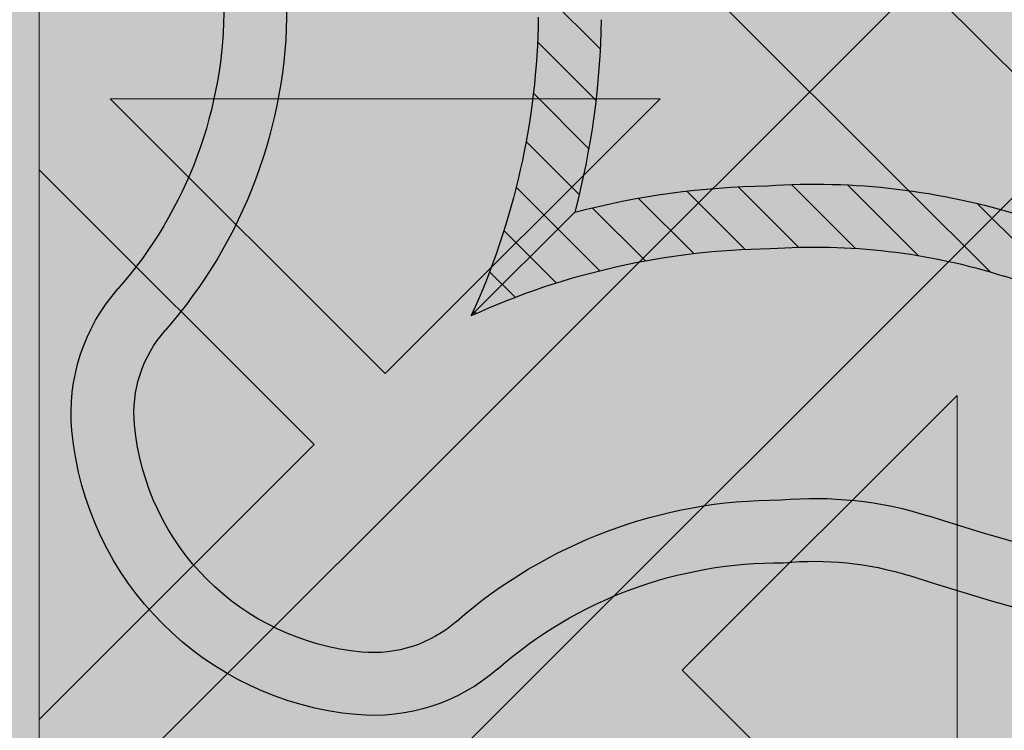
# Model space of a CAD drawing. Units: inches. Extents: x 844 to 2234, y 346 to 1084.
# Tile 28 of 93: x 1252.862 to 1255.358, y 687.38 to 689.183. Entities that reach past the tile are written whole.
import ezdxf

# ---------------------------------------------------------------- set-up
doc = ezdxf.new("R2010")
doc.units = ezdxf.units.IN
doc.header["$MEASUREMENT"] = 0
doc.layers.add('furniture', color=8, linetype='Continuous', lineweight=18)
doc.layers.add('RA-AP-01$0$INT', color=35, linetype='Continuous', lineweight=5)
doc.layers.add('RA-AP-01$0$FURN', color=3, linetype='Continuous')
doc.layers.add('RA-AP-01$0$WOOD', color=64, linetype='Continuous')

# ---------------------------------------------------------------- blocks, each defined once
blk = doc.blocks.new('A$C18D01794')
at = {"layer": 'RA-AP-01$0$INT'}
blk.add_hatch(color=256, dxfattribs=at).paths.add_polyline_path([(4.505206456958071, -6.306712009588038), (5.305206456958072, -6.306712009588038), (5.305206456958072, -7.106712009588038), (5.255206456951893, -7.10671200958804), (5.25520645694868, -6.356712009605972), (4.555206456959269, -6.356712009587461), (4.555206456956052, -7.106712009588038), (4.505206456958073, -7.106712009588038)])
h = blk.add_hatch(color=256, dxfattribs=at)
h.paths.add_polyline_path([(4.585917135068449, -6.356712009588271), (4.555206456959269, -6.35671200958746), (4.555206456959137, -6.387422687716308), (4.874495778835233, -6.706712009592356), (4.90520645695423, -6.676001331474049)])
h.paths.add_polyline_path([(5.255206456948813, -6.387422687716306), (5.255206456948682, -6.356712009605972), (5.224495778822613, -6.356712009605161), (4.905206456953498, -6.676001331474273), (4.935917135072151, -6.706712009592924)])
h.paths.add_polyline_path([(4.935917135072559, -6.706712009592068), (4.905206456953564, -6.737422687710376), (5.255206456951813, -7.087422687708613), (5.255206456951549, -7.026001331471008)])
h.paths.add_polyline_path([(4.555206456956399, -7.026001331471013), (4.555206456956134, -7.087422687708616), (4.905206456953821, -6.737422687710943), (4.874495778835166, -6.70671200959229)])
h = blk.add_hatch(color=256, dxfattribs=at)
h.paths.add_polyline_path([(4.585917135068448, -6.356712009588273), (4.614201406330596, -6.356712009589021), (4.668846067270487, -6.411356670531338), (4.723490728212344, -6.356712009591912), (4.771774999457151, -6.35671200959319), (4.826419660396886, -6.411356670535356), (4.862780050090322, -6.374996280843536), (4.844495778842715, -6.356712009595112), (4.862780050090411, -6.356712009595595), (4.905206456960182, -6.399138416468211), (4.947632863832445, -6.356712009597838), (4.965917135079675, -6.356712009598322), (4.947632863831759, -6.374996280845421), (4.983993253523576, -6.411356670538857), (5.038637914464627, -6.356712009600247), (5.08692218571208, -6.356712009601523), (5.141566846649976, -6.411356670541852), (5.196211507589851, -6.356712009604411), (5.224495778822615, -6.356712009605161), (4.905206456953975, -6.676001331473793)])
h.paths.add_polyline_path([(4.895206456956031, -6.637717060225675), (4.895206456958921, -6.528427738347902), (4.840561796018589, -6.583072399285802)], flags=16)
h.paths.add_polyline_path([(4.915206456955638, -6.637717060226121), (4.969851117895509, -6.583072399288678), (4.915206456957609, -6.528427738348344)], flags=16)
h.paths.add_polyline_path([(4.826419660395175, -6.568930263661755), (4.881064321335613, -6.514285602723745), (4.771774999456703, -6.514285602720857)], flags=16)
h.paths.add_polyline_path([(4.983993253519558, -6.568930263665262), (5.038637914460456, -6.514285602726792), (4.929348592581548, -6.514285602724816)], flags=16)
h.paths.add_polyline_path([(4.881064321336025, -6.494285602723742), (4.826419660397532, -6.439640941782821), (4.771774999457062, -6.494285602720859)], flags=16)
h.paths.add_polyline_path([(4.929348592582019, -6.494285602724817), (5.038637914460982, -6.494285602726792), (4.983993253522945, -6.439640941786327)], flags=16)
h.paths.add_polyline_path([(4.895206456960191, -6.480143467100443), (4.895206456962115, -6.407422687715913), (4.876922185715016, -6.389138416467584), (4.840561796021581, -6.425498806159401)], flags=16)
h.paths.add_polyline_path([(4.915206456958487, -6.480143467100889), (4.969851117899527, -6.425498806162279), (4.933490728206909, -6.389138416468043), (4.9152064569598, -6.40742268771434)], flags=16)
h.paths.add_polyline_path([(4.757632863832376, -6.480143467096812), (4.812277524772842, -6.425498806158772), (4.757632863834348, -6.370854145217844)], flags=16)
h.paths.add_polyline_path([(4.737632863832376, -6.480143467096286), (4.737632863834348, -6.370854145217375), (4.682988202893906, -6.425498806155385)], flags=16)
h.paths.add_polyline_path([(5.05278005008503, -6.480143467103376), (5.052780050087917, -6.370854145224413), (4.998135389146995, -6.425498806162908)], flags=16)
h.paths.add_polyline_path([(5.072780050085024, -6.480143467103744), (5.127424711025931, -6.42549880616527), (5.072780050087916, -6.370854145224832)], flags=16)
h.paths.add_polyline_path([(4.935917135072783, -6.706712009592292), (5.255206456948811, -6.387422687716309), (5.255206456948932, -6.415706958964177), (5.200561796010279, -6.470351619902839), (5.255206456949403, -6.524996280841948), (5.25520645694961, -6.5732805520894), (5.200561796009787, -6.627925213029239), (5.236922185702417, -6.664285602721864), (5.255206456949919, -6.646001331474357), (5.255206456949998, -6.664285602721898), (5.212780050078687, -6.706712009592262), (5.25520645695036, -6.749138416463932), (5.255206456950438, -6.767422687711313), (5.236922185702424, -6.749138416463297), (5.200561796009796, -6.785498806155928), (5.255206456950753, -6.840143467096874), (5.25520645695096, -6.888427738341682), (5.200561796010322, -6.943072399282328), (5.255206456951428, -6.997717060223427), (5.255206456951547, -7.026001331471006)])
h.paths.add_polyline_path([(5.042988202883395, -6.785498806155427), (5.097632863823085, -6.840143467095101), (5.097632863822622, -6.730854145216193)], flags=16)
h.paths.add_polyline_path([(5.028846067259663, -6.771356670531693), (5.083490728198774, -6.716712009592573), (4.974201406321001, -6.716712009593042)], flags=16)
h.paths.add_polyline_path([(5.117632863823087, -6.840143467095186), (5.172277524762331, -6.785498806155926), (5.11763286382262, -6.730854145216225)], flags=16)
h.paths.add_polyline_path([(5.08349072819877, -6.696712009593886), (5.028846067259652, -6.642067348654775), (4.974201406320998, -6.696712009593438)], flags=16)
h.paths.add_polyline_path([(5.131774999446817, -6.854285602718917), (5.186419660386065, -6.799640941779662), (5.241064321325782, -6.854285602719365)], flags=17)
h.paths.add_polyline_path([(5.131774999446228, -6.716712009592374), (5.186419660386065, -6.771356670532194), (5.222780050079488, -6.734996280838764), (5.204495778832781, -6.716712009592063)], flags=16)
h.paths.add_polyline_path([(5.097632863822613, -6.682569873970264), (5.097632863823061, -6.573280552091354), (5.042988202883383, -6.627925213031044)], flags=16)
h.paths.add_polyline_path([(5.131774999446899, -6.874285602718915), (5.241064321325809, -6.874285602719364), (5.186419660386591, -6.928930263658598)], flags=17)
h.paths.add_polyline_path([(5.131774999446226, -6.696712009594078), (5.204495778830767, -6.696712009594374), (5.22278005007868, -6.67842773834687), (5.186419660386049, -6.642067348654249)], flags=16)
h.paths.add_polyline_path([(5.11763286382262, -6.682569873970225), (5.17227752476232, -6.627925213030515), (5.117632863823064, -6.573280552091267)], flags=16)
h.paths.add_polyline_path([(5.186419660386069, -6.613783077405491), (5.241064321325754, -6.559138416465795), (5.131774999446791, -6.559138416466263)], flags=16)
h.paths.add_polyline_path([(5.131774999446872, -6.539138416466263), (5.24106432132578, -6.539138416465794), (5.186419660386554, -6.484493755526573)], flags=16)
h.paths.add_polyline_path([(5.255206456951811, -7.08742268770861), (5.255206456951895, -7.106712009588038), (4.555206456956052, -7.106712009588038), (4.555206456956136, -7.087422687708617), (4.905206456953973, -6.737422687710788)])
h.paths.add_polyline_path([(4.983993253513404, -6.8444937555241), (4.92934859257295, -6.899138416462108), (5.03863791445186, -6.899138416465014)], flags=16)
h.paths.add_polyline_path([(4.969851117889988, -6.83035161990006), (4.915206456952556, -6.775706958960171), (4.915206456949648, -6.884996280837944)], flags=16)
h.paths.add_polyline_path([(4.929348592572535, -6.919138416462105), (4.983993253511019, -6.973783077403037), (5.038637914451496, -6.919138416465012)], flags=16)
h.paths.add_polyline_path([(5.052780050074912, -6.93328055208906), (4.998135389134438, -6.987925213027088), (5.052780050072919, -7.042569873968025)], flags=16)
h.paths.add_polyline_path([(5.07278005007491, -6.933280552089588), (5.072780050072918, -7.042569873968497), (5.127424711013374, -6.987925213030498)], flags=16)
h.paths.add_polyline_path([(4.89520645695295, -6.775706958959721), (4.840561796013067, -6.830351619897157), (4.895206456950961, -6.884996280837494)], flags=16)
h.paths.add_polyline_path([(4.915206456948365, -6.933280552085403), (4.915206456946434, -7.006001331471951), (4.933490728192729, -7.024285602719066), (4.969851117886972, -6.987925213026453)], flags=16)
h.paths.add_polyline_path([(4.881064321327021, -6.899138416461022), (4.82641966038902, -6.84449375552057), (4.771774999448108, -6.899138416459029)], flags=16)
h.paths.add_polyline_path([(4.895206456950073, -6.933280552084951), (4.840561796009022, -6.987925213023558), (4.876922185700835, -7.024285602716997), (4.895206456948749, -7.006001331469487)], flags=16)
h.paths.add_polyline_path([(4.983993253510392, -7.0020673486505), (4.947632863816944, -7.038427738342319), (4.965917135064043, -7.05671200959023), (5.038637914448995, -7.056712009591555)], flags=16)
h.paths.add_polyline_path([(4.881064321326543, -6.91913841646102), (4.771774999447578, -6.919138416459031), (4.826419660385607, -6.973783077399508)], flags=16)
h.paths.add_polyline_path([(4.905206456946447, -7.014285602717636), (4.862780050074785, -7.056712009588352), (4.947632863816685, -7.056712009589775)], flags=16)
h.paths.add_polyline_path([(5.14156684663679, -7.002067348654549), (5.086922185696452, -7.056712009592438), (5.196211507574223, -7.056712009594425)], flags=16)
h.paths.add_polyline_path([(4.8264196603837, -7.002067348646972), (4.771774999442643, -7.056712009585575), (4.8444957788276, -7.056712009587508), (4.862780050075511, -7.038427738340416)], flags=16)
h.paths.add_polyline_path([(4.812277524760289, -6.98792521302292), (4.757632863822258, -6.933280552082447), (4.757632863819352, -7.042569873961408)], flags=16)
h.paths.add_polyline_path([(4.73763286382226, -6.933280552082079), (4.682988202881349, -6.987925213020536), (4.737632863819352, -7.04256987396099)], flags=16)
h.paths.add_polyline_path([(4.723490728195188, -7.056712009584289), (4.668846067257299, -7.002067348643949), (4.614201406317417, -7.056712009581383)], flags=16)
h.paths.add_polyline_path([(4.597632863829262, -6.706712009592262), (4.555206456957951, -6.664285602721896), (4.555206456958029, -6.646001331474357), (4.573490728205535, -6.664285602721864), (4.609851117898167, -6.627925213029238), (4.555206456958338, -6.573280552089402), (4.555206456958546, -6.524996280841952), (4.60985111789767, -6.470351619902839), (4.555206456959015, -6.415706958964177), (4.555206456959138, -6.387422687716309), (4.874495778835167, -6.70671200959229), (4.5552064569564, -7.026001331471015), (4.555206456956523, -6.997717060223433), (4.609851117897629, -6.94307239928233), (4.555206456956988, -6.888427738341681), (4.555206456957198, -6.840143467096881), (4.609851117898153, -6.78549880615593), (4.573490728205528, -6.749138416463297), (4.555206456957507, -6.76742268771132), (4.555206456957585, -6.749138416463933)])
h.paths.add_polyline_path([(4.712780050085332, -6.730854145216195), (4.712780050084863, -6.840143467095105), (4.767424711024555, -6.785498806155427)], flags=16)
h.paths.add_polyline_path([(4.726922185709173, -6.716712009592573), (4.781566846648288, -6.771356670531693), (4.836211507586949, -6.716712009593043)], flags=16)
h.paths.add_polyline_path([(4.692780050085327, -6.730854145216225), (4.638135389145619, -6.785498806155928), (4.692780050084865, -6.840143467095185)], flags=16)
h.paths.add_polyline_path([(4.726922185709182, -6.696712009593886), (4.836211507586949, -6.696712009593436), (4.7815668466483, -6.642067348654773)], flags=16)
h.paths.add_polyline_path([(4.678637914461726, -6.71671200959237), (4.605917135075169, -6.716712009592063), (4.587632863828464, -6.734996280838766), (4.623993253521887, -6.771356670532195)], flags=16)
h.paths.add_polyline_path([(4.712780050085336, -6.68256987397026), (4.767424711024568, -6.627925213031042), (4.71278005008489, -6.573280552091352)], flags=16)
h.paths.add_polyline_path([(4.678637914461726, -6.696712009594076), (4.623993253521899, -6.642067348654247), (4.587632863829271, -6.67842773834687), (4.605917135077185, -6.696712009594376)], flags=16)
h.paths.add_polyline_path([(4.692780050085336, -6.682569873970228), (4.692780050084889, -6.573280552091267), (4.638135389145632, -6.627925213030515)], flags=16)
h.paths.add_polyline_path([(4.623993253521885, -6.799640941779662), (4.678637914461131, -6.854285602718915), (4.56934859258217, -6.854285602719365)], flags=17)
h.paths.add_polyline_path([(4.623993253521901, -6.613783077405509), (4.678637914461158, -6.559138416466263), (4.569348592582195, -6.559138416465795)], flags=16)
h.paths.add_polyline_path([(4.678637914461051, -6.874285602718915), (4.623993253521361, -6.928930263658598), (4.569348592582143, -6.874285602719364)], flags=17)
h.paths.add_polyline_path([(4.678637914461076, -6.539138416466263), (4.623993253521399, -6.484493755526573), (4.569348592582167, -6.539138416465796)], flags=16)
h = blk.add_hatch(color=256, dxfattribs=at)
h.paths.add_polyline_path([(4.969851117891331, -6.583072399286455), (4.915206456952669, -6.63771706022511), (4.915206456952222, -6.528427738347337)])
h.paths.add_polyline_path([(4.895206456953064, -6.637717060225108), (4.840561796014413, -6.583072399286448), (4.895206456953533, -6.528427738347335)])
h.paths.add_polyline_path([(4.826419660390684, -6.568930263662714), (4.771774999451003, -6.514285602723024), (4.881064321329913, -6.514285602723489)])
h.paths.add_polyline_path([(4.881064321329884, -6.494285602723492), (4.771774999450921, -6.494285602723024), (4.82641966039018, -6.439640941783778)])
h.paths.add_polyline_path([(4.895206456953734, -6.48014346709988), (4.840561796013912, -6.425498806160046), (4.876922185707337, -6.389138416466622), (4.895206456954043, -6.40742268771333)])
h.paths.add_polyline_path([(4.862780050082808, -6.374996280843689), (4.826419660390178, -6.411356670536314), (4.771774999450351, -6.356712009596481), (4.844495778835303, -6.356712009596181)])
h.paths.add_polyline_path([(4.812277524766446, -6.425498806160041), (4.757632863827191, -6.480143467099289), (4.757632863826741, -6.370854145220329)])
h.paths.add_polyline_path([(4.737632863827191, -6.480143467099214), (4.682988202887508, -6.425498806159518), (4.737632863826743, -6.370854145220299)])
h.paths.add_polyline_path([(4.668846067263777, -6.41135667053579), (4.614201406325123, -6.356712009597128), (4.723490728202894, -6.356712009596675)])
h.paths.add_polyline_path([(4.905206456953846, -6.399138416467422), (4.862780050082654, -6.356712009596229), (4.947632863824561, -6.356712009595756)])
h.paths.add_polyline_path([(4.915206456952028, -6.480143467099882), (4.91520645695173, -6.407422687715346), (4.933490728199234, -6.389138416467428), (4.96985111789186, -6.425498806160055)])
h.paths.add_polyline_path([(5.038637914454841, -6.494285602723048), (4.929348592575874, -6.494285602723497), (4.983993253515593, -6.439640941783787)])
h.paths.add_polyline_path([(4.983993253515065, -6.568930263662725), (4.929348592575849, -6.514285602723495), (5.038637914454755, -6.514285602723045)])
h.paths.add_polyline_path([(5.052780050079843, -6.480143467099317), (4.998135389140595, -6.425498806160058), (5.052780050080309, -6.370854145220356)])
h.paths.add_polyline_path([(4.983993253516868, -6.411356670536324), (4.947632863824241, -6.374996280843694), (4.965917135071747, -6.356712009596188), (5.038637914456701, -6.356712009596504)])
h.paths.add_polyline_path([(5.127424711019533, -6.425498806159557), (5.072780050079843, -6.480143467099239), (5.07278005008031, -6.370854145220326)])
h.paths.add_polyline_path([(5.141566846643269, -6.411356670535829), (5.086922185704154, -6.356712009596707), (5.196211507581929, -6.356712009597176)])
h = blk.add_hatch(color=256, dxfattribs=at)
h.paths.add_polyline_path([(5.028846067259997, -6.642067348655121), (4.974201406321342, -6.696712009593783), (5.083490728199115, -6.69671200959423)])
h.paths.add_polyline_path([(4.974201406321344, -6.716712009593388), (5.028846067260004, -6.771356670532039), (5.083490728199117, -6.716712009592919)])
h.paths.add_polyline_path([(5.042988202883738, -6.785498806155768), (5.097632863823428, -6.840143467095449), (5.097632863822963, -6.73085414521654)])
h.paths.add_polyline_path([(5.117632863822961, -6.730854145216568), (5.117632863823428, -6.840143467095531), (5.172277524762674, -6.785498806156272)])
h.paths.add_polyline_path([(5.131774999446572, -6.716712009592718), (5.186419660386406, -6.77135667053254), (5.222780050079831, -6.734996280839116), (5.204495778833122, -6.716712009592409)])
h.paths.add_polyline_path([(5.236922185702764, -6.749138416463644), (5.200561796010139, -6.785498806156274), (5.255206456949971, -6.840143467096101), (5.255206456950271, -6.76742268771115)])
h.paths.add_polyline_path([(5.186419660386412, -6.799640941780006), (5.131774999447164, -6.854285602719262), (5.241064321326123, -6.854285602719711)])
h.paths.add_polyline_path([(5.131774999447238, -6.874285602719261), (5.186419660386934, -6.928930263658944), (5.241064321326153, -6.874285602719709)])
h.paths.add_polyline_path([(5.200561796010663, -6.943072399282675), (5.255206456949324, -6.997717060221329), (5.255206456949777, -6.888427738343558)])
h.paths.add_polyline_path([(5.21278005007903, -6.706712009592607), (5.255206456950223, -6.749138416463798), (5.255206456950696, -6.664285602721891)])
h.paths.add_polyline_path([(5.13177499944657, -6.696712009594424), (5.204495778831106, -6.696712009594723), (5.222780050079024, -6.678427738347219), (5.186419660386397, -6.642067348654592)])
h.paths.add_polyline_path([(5.117632863823405, -6.573280552091611), (5.117632863822955, -6.682569873970578), (5.172277524762665, -6.627925213030859)])
h.paths.add_polyline_path([(5.042988202883727, -6.627925213031387), (5.097632863822957, -6.682569873970603), (5.097632863823407, -6.573280552091697)])
h.paths.add_polyline_path([(5.131774999447135, -6.559138416466609), (5.186419660386394, -6.613783077405857), (5.241064321326097, -6.559138416466144)])
h.paths.add_polyline_path([(5.200561796010128, -6.627925213029584), (5.236922185702758, -6.664285602722211), (5.255206456950264, -6.646001331474705), (5.255206456949948, -6.573280552089752)])
h.paths.add_polyline_path([(5.186419660386895, -6.484493755526919), (5.131774999447213, -6.539138416466609), (5.241064321326127, -6.539138416466142)])
h.paths.add_polyline_path([(5.200561796010624, -6.470351619903183), (5.255206456949745, -6.524996280842298), (5.255206456949276, -6.415706958964523)])
for p, q in [((4.905206456953975, -6.676001331473793), (5.224495778822613, -6.356712009605161)), ((5.255206456951895, -7.106712009588038), (5.255206456948681, -6.356712009605972)), ((5.072780050085028, -6.48014346710374), (5.072780050087916, -6.37085414522483)), ((5.072780050087916, -6.37085414522483), (5.127424711025931, -6.42549880616527)), ((4.935917135072783, -6.706712009592292), (5.255206456948813, -6.387422687716307)), ((5.255206456948934, -6.415706958964177), (5.200561796010281, -6.470351619902839)), ((5.12742471102593, -6.425498806165272), (5.072780050085028, -6.48014346710374)), ((5.255206456949399, -6.524996280841946), (5.200561796010281, -6.470351619902839)), ((5.18641966038655, -6.484493755526575), (5.131774999446872, -6.539138416466263)), ((5.241064321325782, -6.539138416465796), (5.186419660386552, -6.484493755526573)), ((5.131774999446872, -6.539138416466263), (5.241064321325782, -6.539138416465796))]:
    blk.add_line(p, q, dxfattribs=at)
blk = doc.blocks.new('A$C32926AE1')
at = {"layer": 'RA-AP-01$0$FURN'}
h = blk.add_hatch(dxfattribs=at)
h.set_pattern_fill('ANSI31', color=256, scale=0.1, style=0)
h.set_pattern_definition([(45, (0, 0), (-0.0088388347648318, 0.0088388347648318), [])])
edge = h.paths.add_edge_path(flags=16)
edge.add_arc((4.904771284329206, 4.246793130718756), 0.2603971832811541, 75.22398030683196, 104.7760196931204)
edge.add_arc((4.904771284329206, 4.246793130718756), 0.2603971832811541, 75.223980306832, 104.77601969312039, ccw=False)
edge = h.paths.add_edge_path(flags=16)
edge.add_arc((4.904771284329206, 4.067062675376612), 0.2603971832811541, 255.2239803068796, 284.776019693168)
edge.add_arc((4.904771284329206, 4.067062675376612), 0.2603971832811541, 255.22398030687958, 284.77601969316805, ccw=False)
edge = h.paths.add_edge_path(flags=0)
edge.add_arc((4.904771284329206, 4.067062675376612), 0.2603971832811541, 255.2239803068796, 284.776019693168)
edge.add_arc((4.904771284329206, 4.067062675376612), 0.2603971832811541, 255.22398030687958, 284.77601969316805, ccw=False)
edge = h.paths.add_edge_path(flags=0)
edge.add_arc((4.904771284329206, 4.067062675376612), 0.2603971832811541, 255.2239803068796, 284.776019693168)
edge.add_arc((4.904771284329206, 4.067062675376612), 0.2603971832811541, 255.22398030687958, 284.77601969316805, ccw=False)
edge = h.paths.add_edge_path()
edge.add_arc((4.604388392048174, 4.588829985554312), 0.1599999999999918, 342.3781640246255, 354.4317409793762)
edge.add_arc((5.090145208887507, 4.43216705527679), 0.3503971832811637, 162.0091218307731, 180.3186872093483)
edge.add_arc((5.205154176610243, 4.588829985554953), 0.1599999999999917, 185.5682590208461, 197.6218359767349)
edge.add_arc((4.904771284329229, 4.246793130718735), 0.3503971832811761, 72.00912183053516, 107.9908781690354)
edge.add_arc((9.535952835716557, 4.28682295566602), 4.798342501046485, 178.2875002453811, 181.5576802719453)
edge.add_arc((4.719397359771122, 4.43216705527679), 0.3503971832811637, 359.6813127906516, 377.9908781692269)
edge.add_arc((9.535967292294904, 4.286822350292874), 4.778371420254705, 178.2965938931842, 181.5667745797229)
edge.add_arc((4.719397359771122, 4.43216705527679), 0.3303971832811637, 359.6813127906516, 377.9908781692269)
edge.add_arc((0.2735752763637294, 4.286822350292874), 4.7783714202547, 358.4332254202771, 361.7034061068158)
edge.add_arc((5.061434214606998, 4.732549947558029), 0.1600000000000254, 252.3781640250584, 264.4317409792362)
edge.add_arc((4.748108354051257, 4.732549947558012), 0.1600000000000541, 275.5682590208426, 287.6218359759532)
edge.add_arc((4.604388392048115, 4.588829985554317), 0.1800000000000505, 342.3567572500182, 349.3735009646207)
edge.add_arc((5.205154176610254, 4.588829985554976), 0.1800000000000069, 190.6264990356027, 197.6432427513933)
edge.add_arc((5.061434214607106, 4.732549947558013), 0.1800000000000424, 252.3567572496606, 259.3735009644582)
edge.add_arc((4.904771284329208, 4.246793130718737), 0.3303971832811676, 71.99844483668534, 108.0015551637021)
edge.add_arc((4.748108354051414, 4.732549947558045), 0.1800000000000547, 280.6264990355479, 287.6432427495938)
edge.add_arc((5.090145208887514, 4.432167055276789), 0.2803971832811691, 162.8706300666893, 180.816523289902)
edge.add_arc((4.719397359771136, 4.432167055276689), 0.2803971832811534, 359.183476710103, 377.1293699333214)
edge.add_arc((4.904771284329222, 4.246793130718737), 0.2803971832811769, 72.87063006672916, 107.1293699332334)
edge.add_arc((5.090145208887522, 4.432167055276788), 0.2603971832811776, 165.2239803068007, 180.9953123810312)
edge.add_arc((4.719397359771141, 4.432167055276699), 0.2603971832811458, 359.0046876189768, 374.7760196932087)
edge.add_arc((5.090145208887507, 4.43216705527679), 0.3303971832811637, 162.0091218307731, 180.3186872093483)
edge.add_arc((9.53595427642584, 4.285015535491528), 4.728345371032053, 178.265043920078, 181.5679956281801)
edge.add_arc((0.2735882922327999, 4.285015535491582), 4.728345371032045, 358.4320043718193, 361.7349560799204)
edge.add_arc((9.535953591267507, 4.284458026472751), 4.708343996644348, 178.2573054306777, 181.5704995759608)
edge.add_arc((0.273588977391114, 4.284458026472785), 4.708343996644358, 358.4295004240388, 361.7426945693213)
edge.add_arc((0.2735889773911131, 4.029397779622582), 4.708343996644359, 358.2573054306787, 361.5704995759613)
edge.add_arc((9.535953591267518, 4.029397779622618), 4.708343996644359, 178.4295004240391, 181.7426945693223)
edge.add_arc((0.2735882922327901, 4.028840270603786), 4.728345371032054, 358.2650439200796, 361.5679956281808)
edge.add_arc((9.53595427642584, 4.028840270603841), 4.728345371032054, 178.4320043718199, 181.7349560799219)
edge.add_arc((0.2735752763637302, 4.027033455802493), 4.778371420254699, 358.2965938931842, 361.5667745797229)
edge.add_arc((4.719397359771122, 3.881688750818578), 0.3303971832811637, 342.0091218307731, 360.3186872093484)
edge.add_arc((5.090145208887507, 3.881688750818578), 0.3303971832811637, 179.6813127906516, 197.9908781692269)
edge.add_arc((9.535967292294904, 4.027033455802493), 4.778371420254705, 178.433225420277, 181.7034061068158)
edge.add_arc((4.719397359771122, 3.881688750818578), 0.3503971832811637, 342.0091218307731, 360.3186872093484)
edge.add_arc((9.53595283571655, 4.027032850429349), 4.79834250104648, 178.4423197280546, 181.7124997546188)
edge.add_arc((4.719397359771141, 3.881688750818669), 0.2603971832811458, 345.2239803067913, 360.9953123810232)
edge.add_arc((5.090145208887522, 3.88168875081858), 0.2603971832811776, 179.0046876189687, 194.7760196931993)
edge.add_arc((4.904771284329222, 4.067062675376631), 0.2803971832811769, 252.8706300667665, 287.1293699332708)
edge.add_arc((4.719397359771136, 3.881688750818678), 0.2803971832811534, 342.8706300666787, 360.8165232898969)
edge.add_arc((5.090145208887514, 3.881688750818579), 0.2803971832811691, 179.183476710098, 197.1293699333106)
edge.add_arc((4.748108354051414, 3.581305858537323), 0.1800000000000547, 72.3567572504062, 79.37350096445199)
edge.add_arc((4.904771284329208, 4.067062675376631), 0.3303971832811676, 251.9984448362979, 288.0015551633146)
edge.add_arc((5.061434214607106, 3.581305858537355), 0.1800000000000424, 100.6264990355418, 107.6432427503394)
edge.add_arc((5.205154176610254, 3.725025820540392), 0.1800000000000069, 162.3567572486066, 169.3735009643972)
edge.add_arc((4.604388392048115, 3.725025820541051), 0.1800000000000505, 10.62649903537925, 17.64324274998182)
edge.add_arc((4.748108354051257, 3.581305858537356), 0.1600000000000541, 72.37816402404681, 84.43174097915735)
edge.add_arc((4.904771284329229, 4.067062675376632), 0.3503971832811761, 252.0091218309645, 287.9908781694648)
edge.add_arc((5.061434214606998, 3.581305858537339), 0.1600000000000254, 95.56825902076373, 107.6218359749416)
edge.add_arc((5.205154176610243, 3.725025820540414), 0.1599999999999917, 162.3781640232651, 174.4317409791539)
edge.add_arc((5.090145208887507, 3.881688750818578), 0.3503971832811637, 179.6813127906516, 197.9908781692269)
edge.add_arc((4.604388392048174, 3.725025820541056), 0.1599999999999918, 5.568259020623824, 17.62183597537444)
edge.add_arc((0.2735897329420762, 4.28682295566602), 4.798342501046482, 358.4423197280547, 361.7124997546188)
edge.add_arc((0.2735897329420691, 4.027032850429348), 4.798342501046489, 358.2875002453812, 361.5576802719453)
at = {"layer": 'RA-AP-01$0$WOOD'}
h = blk.add_hatch(color=256, dxfattribs=at)
h.dxf.hatch_style = 1
h.paths.add_polyline_path([(5.157430609644524, 4.573483066760929, -0.1009492694046607), (5.155401577623758, 4.593365984175333, -0.1842662638101597), (5.172249623284174, 4.638795604568598, 0.2056608120311276), (5.179560981299304, 4.661316324430096, 0.3614336704623542), (5.134352340494423, 4.706524965234944, 0.2056608120311297), (5.111831620632933, 4.699213607219793, -0.1842662638101113), (5.066402000239693, 4.682365561559342, -0.1055311479399994), (5.045656153913092, 4.68467289944697, 0.1567636581983829), (4.763886414745334, 4.684672899446966, -0.1055311479399895), (4.743140568418733, 4.68236556155934, -0.1842662638100833), (4.6977109480255, 4.69921360721979, 0.2056608120302612), (4.675190228164109, 4.706524965234949, 0.3614336704708441), (4.629981587358889, 4.66131632442871, 0.2056608120245944), (4.637292945374126, 4.638795604567974, -0.1842662638101024), (4.654140991034615, 4.59336598417475, -0.1009492694055169), (4.652111959013835, 4.573483066760181, 0.021410119221476), (4.629748025606143, 4.156712009541676, 0.0214101192214795), (4.652111959013809, 3.739940952323101, -0.1009492694059586), (4.654140991034615, 3.720058034908448, -0.1842662638100975), (4.637292945374126, 3.674628414515226, 0.2056608120245705), (4.629981587358889, 3.652107694654492, 0.3614336704708879), (4.675190228164113, 3.606899053848249, 0.2056608120302384), (4.697710948025501, 3.614210411863408, -0.1842662638100995), (4.743140568418738, 3.63105845752386, -0.1055311479402541), (4.763886414745388, 3.628751119636215, 0.1567636581983776), (5.045656153913137, 3.628751119636244, -0.1055311479397538), (5.066402000239692, 3.631058457523857, -0.1842662638101067), (5.111831620632931, 3.614210411863407, 0.2056608120310924), (5.134352340494417, 3.606899053848256, 0.3614336704624001), (5.179560981299307, 3.652107694653103, 0.2056608120311314), (5.172249623284175, 3.6746284145146, -0.1842662638101402), (5.155401577623758, 3.72005803490786, -0.1009492694051366), (5.15743060964455, 3.739940952322354, 0.0214101192215073), (5.179794543052287, 4.156712009541468, 0.0214101192215252)])
h.paths.add_polyline_path([(4.639748609479751, 4.156712009541513, 0.0213537860821624), (4.661970494867118, 3.741887061152232, -0.094075836301374), (4.664143710413708, 3.7196126951003, -0.1824818158568985), (4.644813765429836, 3.668037719127816, 0.2056608120245319), (4.639939526753007, 3.653023905887301, 0.3614336704710246), (4.676106439397173, 3.616856993242342, 0.2056608120302234), (4.691120252638095, 3.621731231919122, -0.1824818158602558), (4.742695228611606, 3.641061176902986, -0.1029891339458722), (4.766991894714349, 3.638256818950944, 0.156709409989566), (5.042550673941472, 3.638256818950105, -0.102989133958497), (5.066847340047078, 3.641061176902949, -0.1824818158594995), (5.118422316020358, 3.621731231919103, 0.2056608120311416), (5.133436129261316, 3.616856993242346, 0.3614336704621468), (5.169603041905217, 3.653023905886178, 0.2056608120310986), (5.164728803228477, 3.668037719127177, -0.1824818158565612), (5.145398858244737, 3.719612695099578, -0.0940758363009313), (5.147572073791232, 3.741887061151398, 0.0213537860822023), (5.169793959178681, 4.156712009541451, 0.0213537860822226), (5.147572073791203, 4.571536957931898, -0.0940758363005034), (5.145398858244737, 4.59381132398362, -0.1824818158565587), (5.164728803228476, 4.645386299956021, 0.2056608120311045), (5.169603041905216, 4.66040011319702, 0.3614336704621845), (5.133436129261313, 4.696567025840856, 0.2056608120310773), (5.118422316020359, 4.691692787164098, -0.182481815859508), (5.066847340047078, 4.67236284218025, -0.1029891339584606), (5.04255067394148, 4.675167200133092, 0.156709409989566), (4.766991894714357, 4.675167200132257, -0.1029891339458842), (4.742695228611611, 4.672362842180213, -0.1824818158602725), (4.691120252638095, 4.691692787164077, 0.2056608120302152), (4.676106439397174, 4.696567025840858, 0.3614336704710363), (4.639939526753005, 4.660400113195899, 0.2056608120245495), (4.644813765429837, 4.645386299955384, -0.1824818158568934), (4.664143710413708, 4.593811323982902, -0.0940758363009187), (4.661970494867149, 4.571536957931074, 0.021353786082177)], flags=16)
h.paths.add_polyline_path([(5.129794543052235, 4.432167055276933, -0.0141661062790638), (5.130152669293814, 4.156927903047693, -0.0141661062790647), (5.129794543052234, 3.881688750818433, -0.0785247771143638), (5.10979738006795, 3.755143611847103, 0.0945969212073497), (5.105408519571111, 3.717898134952927, 0.1043170707844957), (5.116074640131521, 3.670385395016088, 0.1043170707864965), (5.068561900193738, 3.681051515576561, 0.09459692119553), (5.031316423304057, 3.676662655080835, -0.1580239521427272), (4.778226145355827, 3.676662655080367, 0.0945969211986668), (4.740980668464973, 3.681051515576592, 0.1043170707882822), (4.693467928526415, 3.670385395015844, 0.1043170707867916), (4.704134049087309, 3.717898134953662, 0.0945969211972894), (4.69974518859162, 3.755143611844042, -0.0785247771163196), (4.679748025606343, 3.881688750818406, -0.0141661062790663), (4.679389899364763, 4.156927903047693, -0.0141661062790672), (4.679748025606343, 4.432167055276998, -0.0785247771163064), (4.699745188591625, 4.55871219425134, 0.094596921197333), (4.704134049087308, 4.595957671141738, 0.1043170707867205), (4.693467928526416, 4.643470411079523, 0.1043170707882628), (4.740980668464965, 4.632804290518776, 0.0945969211988114), (4.778226145355874, 4.637193151015016, -0.158023952142669), (5.031316423304015, 4.637193151014546, 0.0945969211956361), (5.068561900193736, 4.632804290518806, 0.1043170707864979), (5.11607464013152, 4.643470411079278, 0.1043170707844617), (5.105408519571112, 4.595957671142455, 0.0945969212074597), (5.109797380067959, 4.558712194248236, -0.0785247771143467)], flags=0)
h.paths.add_polyline_path([(5.119794532311105, 4.432259799204851, -0.0142000800617244), (5.120156169157484, 4.156927903047701, -0.0142000800617277), (5.119794532311105, 3.881596006890482, -0.0784894509520253), (5.100273383573699, 3.758192358677797, 0.0940138827242913), (5.095413455884425, 3.717477693979438, 0.0606271852308753), (5.099615656341024, 3.686844378806616, 0.0606271852322524), (5.068982341167493, 3.691046579263239, 0.0940138827010453), (5.028267676478798, 3.686186651576848, -0.1580706864508061), (4.781274892180912, 3.686186651576435, 0.0940138827026903), (4.740560227491556, 3.691046579263279, 0.0606271852339895), (4.709926912317155, 3.686844378806508, 0.0606271852329405), (4.714129112773991, 3.717477693980356, 0.094013882701304), (4.709269185087677, 3.758192358669163, -0.0784894509577193), (4.689748036347473, 3.881596006890469, -0.014200080061729), (4.689386399501094, 4.156927903047709, -0.0142000800617217), (4.689748036347473, 4.432259799204808, -0.078489450957724), (4.709269185087651, 4.555663447426125, 0.0940138827014585), (4.714129112773992, 4.596378112114996, 0.0606271852329731), (4.709926912317154, 4.62701142728886, 0.0606271852340196), (4.74056022749157, 4.622809226832087, 0.0940138827024997), (4.781274892180847, 4.627669154518912, -0.1580706864508359), (5.028267676478777, 4.627669154518526, 0.0940138827010946), (5.068982341167492, 4.622809226832129, 0.060627185232254), (5.099615656341024, 4.627011427288751, 0.0606271852308727), (5.095413455884425, 4.59637811211593, 0.0940138827241088), (5.100273383573675, 4.555663447417647, -0.0784894509520978)], flags=0)
h.paths.add_polyline_path([(5.06978912287499, 4.430218106756144, -0.014241683694547), (5.070173729147532, 4.156927903047672, -0.0142416836945458), (5.06978912287499, 3.883637699339223, -0.0800609523125196), (5.052662118612511, 3.773463122773442, 0.0526421978001116), (5.04590916754064, 3.740550867606997, 0.0526421977992423), (5.012996912374707, 3.73379791653534, -0.1583028414718258), (4.796545656286308, 3.73379791653451, 0.0526421978034211), (4.763633401117837, 3.740550867607021, 0.0526421978018622), (4.756880450045755, 3.773463122774558, -0.0800609523117106), (4.739753445783639, 3.883637699339268, -0.0142416836945435), (4.739368839511098, 4.156927903047671, -0.0142416836945477), (4.739753445783639, 4.430218106756155, -0.0800609523116345), (4.75688045004574, 4.540392683320762, 0.052642197801941), (4.763633401117837, 4.573304938488346, 0.0526421978035071), (4.796545656286361, 4.580057889560873, -0.1583028414717561), (5.012996912374669, 4.580057889560039, 0.0526421977993048), (5.04590916754064, 4.57330493848837, 0.0526421978002057), (5.052662118612529, 4.540392683321868, -0.080060952312477)], flags=0)
h.paths.add_polyline_path([(5.049789715110557, 4.43038092723357, -0.0143097550741839), (5.05018085590259, 4.156927903047715, -0.0143097550741854), (5.049789715110558, 3.883474878861827, -0.0800685599149176), (5.03362098255317, 3.779581877367999, 0.0306258898956367), (5.028241146483733, 3.758218888663947, 0.0306258898977031), (5.006878157778253, 3.75283905259408, -0.1583983521624096), (4.802664410878162, 3.752839052594731, 0.0306258898946014), (4.781301422174808, 3.758218888663924, 0.0306258898967912), (4.775921586105202, 3.779581877368794, -0.080068559914251), (4.759752853548071, 3.883474878861786, -0.0143097550741854), (4.759361712756037, 4.156927903047671, -0.0143097550741854), (4.759752853548071, 4.430380927233557, -0.0800685599142479), (4.775921586105193, 4.534273928726546, 0.0306258898968306), (4.781301422174808, 4.555636917431444, 0.0306258898945754), (4.802664410878143, 4.561016753500631, -0.1583983521624168), (5.006878157778244, 4.561016753501291, 0.0306258898977177), (5.028241146483733, 4.555636917431421, 0.0306258898958182), (5.03362098255321, 4.534273928727244, -0.080068559914796)], flags=0)
h.paths.add_polyline_path([(4.999766070382627, 4.428171244713864, -0.0143443147609634), (5.000198441819402, 4.156927903047689, -0.0143443147609612), (4.999766070382627, 3.885684561381556, -0.0784641635803329), (4.987356730658798, 3.799103304488872, -0.1506053783831347), (4.822185837999821, 3.79910330448882, -0.0784641635803318), (4.809776498276007, 3.885684561381509, -0.014344314760963), (4.809344126839227, 4.156927903047677, -0.0143443147609645), (4.809776498276007, 4.428171244713873, -0.0784641635803192), (4.822185837999822, 4.514752501606549, -0.1506053783831338), (4.987356730658798, 4.514752501606494, -0.078464163580285)], flags=0)
h.paths.add_polyline_path([(4.979755254238824, 4.42764379880488, -0.0143772539198268), (4.980205517789977, 4.156927903047693, -0.0143772539198275), (4.979755254238824, 3.886212007290489, -0.0689242507424422), (4.971183264704897, 3.815276770442801, -0.1296645318904179), (4.838359303953726, 3.815276770442746, -0.0689242507424186), (4.829787314419809, 3.886212007290419, -0.0143772539198292), (4.829337050868653, 4.156927903047653, -0.0143772539198325), (4.829787314419809, 4.427643798804946, -0.0689242507424211), (4.838359303953725, 4.498579035652621, -0.1296645318904187), (4.971183264704897, 4.498579035652565, -0.0689242507424401)], flags=0)
h = blk.add_hatch(color=256, dxfattribs=at)
h.dxf.hatch_style = 1
h.paths.add_polyline_path([(5.145398858244737, 4.59381132398362, -0.1824818158565616), (5.164728803228476, 4.645386299956021, 0.2056608120311045), (5.169603041905216, 4.66040011319702, 0.3614336704621845), (5.133436129261313, 4.696567025840856, 0.2056608120310773), (5.118422316020359, 4.691692787164098, -0.182481815859508), (5.066847340047078, 4.67236284218025, -0.1029891339584606), (5.04255067394148, 4.675167200133092, 0.156709409989566), (4.766991894714357, 4.675167200132257, -0.1029891339458842), (4.742695228611611, 4.672362842180213, -0.1824818158602725), (4.691120252638095, 4.691692787164077, 0.2056608120302152), (4.676106439397174, 4.696567025840858, 0.3614336704710363), (4.639939526753005, 4.660400113195899, 0.2056608120245495), (4.644813765429837, 4.645386299955384, -0.1824818158568934), (4.664143710413708, 4.593811323982902, -0.0940758363009187), (4.661970494867149, 4.571536957931074, 0.0213537860821772), (4.639748609479751, 4.156712009541507, 0.0213537860821625), (4.661970494867119, 3.741887061152226, -0.0940758363013071), (4.664143710413708, 3.719612695100309, -0.1824818158569294), (4.644813765429836, 3.668037719127816, 0.2056608120245319), (4.639939526753007, 3.653023905887301, 0.3614336704710246), (4.676106439397173, 3.616856993242342, 0.2056608120302234), (4.691120252638095, 3.621731231919122, -0.1824818158602558), (4.742695228611606, 3.641061176902986, -0.1029891339458722), (4.766991894714349, 3.638256818950944, 0.156709409989566), (5.042550673941472, 3.638256818950105, -0.102989133958497), (5.066847340047078, 3.641061176902949, -0.1824818158594995), (5.118422316020358, 3.621731231919103, 0.2056608120311416), (5.133436129261316, 3.616856993242346, 0.3614336704621468), (5.169603041905217, 3.653023905886178, 0.2056608120310986), (5.164728803228477, 3.668037719127177, -0.1824818158565612), (5.145398858244737, 3.719612695099578, -0.0940758363009313), (5.147572073791232, 3.741887061151398, 0.0213537860822023), (5.169793959178681, 4.156712009541451, 0.0213537860822226), (5.147572073791203, 4.571536957931898, -0.0940758363004996)])
h.paths.add_polyline_path([(5.109797380067958, 4.55871219424824, -0.0785247771143472), (5.129794543052234, 4.432167055276936, -0.0141661062790644), (5.130152669293814, 4.156927903047685, -0.014166106279066), (5.129794543052234, 3.881688750818401, -0.0785247771143517), (5.109797380067946, 3.755143611847092, 0.0945969212073132), (5.105408519571111, 3.717898134952929, 0.1043170707844995), (5.116074640131521, 3.670385395016088, 0.1043170707864965), (5.068561900193738, 3.681051515576561, 0.09459692119553), (5.031316423304057, 3.676662655080835, -0.1580239521427272), (4.778226145355827, 3.676662655080367, 0.0945969211986668), (4.740980668464973, 3.681051515576592, 0.1043170707882822), (4.693467928526415, 3.670385395015844, 0.1043170707867916), (4.704134049087309, 3.717898134953662, 0.0945969211972894), (4.69974518859162, 3.755143611844042, -0.0785247771163196), (4.679748025606343, 3.881688750818406, -0.0141661062790663), (4.679389899364763, 4.156927903047693, -0.0141661062790672), (4.679748025606343, 4.432167055276998, -0.0785247771163064), (4.699745188591625, 4.55871219425134, 0.094596921197333), (4.704134049087308, 4.595957671141738, 0.1043170707867205), (4.693467928526416, 4.643470411079523, 0.1043170707882628), (4.740980668464965, 4.632804290518776, 0.0945969211988114), (4.778226145355874, 4.637193151015016, -0.158023952142669), (5.031316423304015, 4.637193151014546, 0.0945969211956361), (5.068561900193736, 4.632804290518806, 0.1043170707864979), (5.11607464013152, 4.643470411079278, 0.1043170707844617), (5.105408519571112, 4.595957671142455, 0.0945969212074504)], flags=16)
h.paths.add_polyline_path([(5.100273383573655, 4.55566344741771, -0.0784894509521388), (5.119794532311105, 4.432259799204852, -0.0142000800617252), (5.120156169157484, 4.156927903047686, -0.014200080061726), (5.119794532311105, 3.881596006890502, -0.0784894509520446), (5.100273383573696, 3.758192358677786, 0.0940138827242721), (5.095413455884425, 3.717477693979436, 0.0606271852308692), (5.099615656341024, 3.686844378806616, 0.0606271852322522), (5.068982341167493, 3.691046579263239, 0.0940138827010453), (5.028267676478798, 3.686186651576848, -0.1580706864508061), (4.781274892180912, 3.686186651576435, 0.0940138827026903), (4.740560227491556, 3.691046579263279, 0.0606271852339895), (4.709926912317155, 3.686844378806508, 0.0606271852329405), (4.714129112773991, 3.717477693980356, 0.094013882701304), (4.709269185087677, 3.758192358669163, -0.0784894509577193), (4.689748036347473, 3.881596006890469, -0.014200080061729), (4.689386399501094, 4.156927903047709, -0.0142000800617217), (4.689748036347473, 4.432259799204808, -0.078489450957724), (4.709269185087651, 4.555663447426125, 0.0940138827014585), (4.714129112773992, 4.596378112114996, 0.0606271852329731), (4.709926912317154, 4.62701142728886, 0.0606271852340196), (4.74056022749157, 4.622809226832087, 0.0940138827024997), (4.781274892180847, 4.627669154518912, -0.1580706864508359), (5.028267676478777, 4.627669154518526, 0.0940138827010946), (5.068982341167492, 4.622809226832129, 0.060627185232254), (5.099615656341024, 4.627011427288751, 0.0606271852308727), (5.095413455884425, 4.59637811211593, 0.094013882723957)], flags=0)
h.paths.add_polyline_path([(5.04590916754064, 4.57330493848837, 0.0526421978002057), (5.052662118612529, 4.540392683321868, -0.0800609523124783), (5.06978912287499, 4.430218106756142, -0.0142416836945469), (5.070173729147532, 4.156927903047672, -0.0142416836945458), (5.06978912287499, 3.883637699339223, -0.0800609523125196), (5.052662118612511, 3.773463122773442, 0.0526421978001116), (5.04590916754064, 3.740550867606997, 0.0526421977992423), (5.012996912374707, 3.73379791653534, -0.1583028414718258), (4.796545656286308, 3.73379791653451, 0.0526421978034211), (4.763633401117837, 3.740550867607021, 0.0526421978018622), (4.756880450045755, 3.773463122774558, -0.0800609523117106), (4.739753445783639, 3.883637699339268, -0.0142416836945435), (4.739368839511098, 4.156927903047671, -0.0142416836945477), (4.739753445783639, 4.430218106756155, -0.0800609523116345), (4.75688045004574, 4.540392683320762, 0.052642197801941), (4.763633401117837, 4.573304938488346, 0.0526421978035071), (4.796545656286361, 4.580057889560873, -0.1583028414717561), (5.012996912374669, 4.580057889560039, 0.0526421977993048)], flags=0)
h.paths.add_polyline_path([(5.028241146483733, 4.555636917431422, 0.0306258898956949), (5.033620982553182, 4.534273928727329, -0.0800685599148649), (5.049789715110557, 4.430380927233569, -0.0143097550741839), (5.05018085590259, 4.156927903047715, -0.0143097550741854), (5.049789715110558, 3.883474878861827, -0.0800685599149176), (5.03362098255317, 3.779581877367999, 0.0306258898956367), (5.028241146483733, 3.758218888663947, 0.0306258898977031), (5.006878157778253, 3.75283905259408, -0.1583983521624096), (4.802664410878162, 3.752839052594731, 0.0306258898946014), (4.781301422174808, 3.758218888663924, 0.0306258898967912), (4.775921586105202, 3.779581877368794, -0.080068559914251), (4.759752853548071, 3.883474878861786, -0.0143097550741854), (4.759361712756037, 4.156927903047671, -0.0143097550741854), (4.759752853548071, 4.430380927233557, -0.0800685599142479), (4.775921586105193, 4.534273928726546, 0.0306258898968306), (4.781301422174808, 4.555636917431444, 0.0306258898945754), (4.802664410878143, 4.561016753500631, -0.1583983521624168), (5.006878157778244, 4.561016753501291, 0.0306258898977174)], flags=0)
h.paths.add_polyline_path([(4.987356730658798, 4.514752501606494, -0.0784641635803018), (4.999766070382627, 4.428171244713845, -0.0143443147609637), (5.000198441819402, 4.156927903047665, -0.0143443147609622), (4.999766070382628, 3.885684561381514, -0.0784641635802952), (4.987356730658797, 3.799103304488872, -0.1506053783831338), (4.822185837999821, 3.799103304488819, -0.0784641635803342), (4.809776498276007, 3.885684561381512, -0.0143443147609628), (4.809344126839227, 4.156927903047676, -0.0143443147609646), (4.809776498276007, 4.428171244713873, -0.0784641635803192), (4.822185837999822, 4.514752501606549, -0.1506053783831338)], flags=0)
h.paths.add_polyline_path([(4.971183264704897, 4.498579035652566, -0.0689242507424384), (4.979755254238824, 4.427643798804883, -0.0143772539198276), (4.980205517789977, 4.15692790304768, -0.0143772539198258), (4.979755254238823, 3.88621200729051, -0.0689242507424628), (4.971183264704897, 3.815276770442801, -0.129664531890417), (4.838359303953726, 3.815276770442746, -0.0689242507424186), (4.829787314419809, 3.886212007290419, -0.0143772539198292), (4.829337050868653, 4.156927903047653, -0.0143772539198325), (4.829787314419809, 4.427643798804946, -0.0689242507424211), (4.838359303953725, 4.498579035652621, -0.1296645318904187)], flags=0)
h = blk.add_hatch(dxfattribs=at)
h.set_pattern_fill('ANSI31', color=256, scale=0.05, style=0)
h.set_pattern_definition([(45, (0, 0), (-0.0044194173824159, 0.0044194173824159), [])])
h.paths.add_polyline_path([(5.130152669293814, 4.156927903047704, 0.0141661062790657), (5.129794543052234, 4.432167055276982, 0.0777827904001433), (5.110168979996553, 4.557559993161921, -0.0976515123401879), (5.105408519571111, 4.595957671142454, -0.1043170707844687), (5.116074640131522, 4.64347041107928), (5.099615656341024, 4.627011427288751, 0.0606271852308727), (5.095413455884425, 4.59637811211593, 0.0940138827241088), (5.100273383573675, 4.555663447417647, -0.0784894509520972), (5.119794532311105, 4.432259799204852, -0.0142000800617252), (5.120156169157484, 4.156927903047686, -0.014200080061726), (5.119794532311105, 3.881596006890502, -0.0784894509520446), (5.100273383573696, 3.758192358677786, 0.0940138827242721), (5.095413455884425, 3.717477693979436, 0.0606271852308692), (5.099615656341024, 3.686844378806616), (5.116074640131519, 3.67038539501609, -0.1043170707844594), (5.105408519571112, 3.717898134952912, -0.0976515123401594), (5.11016897999655, 3.756295812933435, 0.0777827904001654), (5.129794543052234, 3.881688750818409, 0.0141661062790665)])
h.paths.add_polyline_path([(5.030164222210597, 3.676291055149937, -0.0976515123472002), (5.068561900193739, 3.681051515576561, -0.1043170707864927), (5.116074640131521, 3.670385395016088), (5.099615656341024, 3.686844378806616, 0.0606271852322522), (5.068982341167493, 3.691046579263239, 0.0940138827010453), (5.028267676478798, 3.686186651576848, -0.1580706864508061), (4.781274892180912, 3.686186651576435, 0.0940138827026903), (4.740560227491556, 3.691046579263279, 0.0606271852339913), (4.709926912317154, 3.686844378806508), (4.693467928526416, 3.670385395015845, -0.1043170707882796), (4.740980668464973, 3.681051515576592, -0.0976515123427246), (4.779378346446416, 3.676291055150394, 0.156512506893803)])
h.paths.add_polyline_path([(4.689748036347473, 3.881596006890472, -0.014200080061729), (4.689386399501094, 4.156927903047712, -0.0142000800617195), (4.689748036347473, 4.432259799204768, -0.078489450957742), (4.709269185087648, 4.555663447426114, 0.0940138827014821), (4.714129112773992, 4.596378112114995, 0.0606271852329748), (4.709926912317154, 4.62701142728886), (4.693467928526414, 4.643470411079524, -0.1043170707867939), (4.704134049087309, 4.595957671141706, -0.09765151234893), (4.699373588660725, 4.557559993157876, 0.0777827903975372), (4.679748025606343, 4.432167055276987, 0.0141661062790675), (4.679389899364763, 4.156927903047675, 0.0141661062790641), (4.679748025606343, 3.88168875081843, 0.0777827903975637), (4.699373588660724, 3.756295812937497, -0.0976515123490278), (4.704134049087308, 3.717898134953629, -0.1043170707867196), (4.693467928526416, 3.670385395015845), (4.709926912317155, 3.686844378806508, 0.0606271852329413), (4.714129112773991, 3.717477693980357, 0.0940138827013084), (4.709269185087676, 3.758192358669166, -0.0784894509577192)])
h.paths.add_polyline_path([(4.779378346446434, 4.63756475094498, -0.0976515123427943), (4.740980668464964, 4.632804290518776, -0.1043170707882609), (4.693467928526416, 4.643470411079523), (4.709926912317154, 4.62701142728886, 0.0606271852340196), (4.74056022749157, 4.622809226832087, 0.0940138827024997), (4.781274892180847, 4.627669154518912, -0.1580706864508359), (5.028267676478777, 4.627669154518526, 0.0940138827010946), (5.068982341167492, 4.622809226832129, 0.060627185232254), (5.099615656341024, 4.627011427288751), (5.116074640131521, 4.643470411079279, -0.1043170707865022), (5.068561900193735, 4.632804290518806, -0.0976515123475899), (5.030164222210446, 4.637564750945479, 0.1565125068936924)])
h = blk.add_hatch(dxfattribs=at)
h.set_pattern_fill('ANSI32', color=256, scale=0.2, style=0)
h.set_pattern_definition([(45, (0, 0), (-0.0530330085889911, 0.0530330085889911), []), (45, (0.035355339, 0), (-0.0530330085889911, 0.0530330085889911), [])])
h.paths.add_polyline_path([(5.119794532311105, 4.432259799204823, 0.0777015974868765), (5.10065834347252, 4.554469821747928, -0.0968902511992216), (5.095413455884425, 4.596378112115931, -0.060627185230871), (5.099615656341024, 4.627011427288751, -0.060627185232254), (5.068982341167492, 4.622809226832129, -0.0968902512198245), (5.027074050790956, 4.628054114423209, 0.1564657949319105), (4.782468517866163, 4.628054114422785, -0.0968902512152247), (4.740560227491555, 4.622809226832088, -0.0606271852339878), (4.709926912317155, 4.627011427288859, -0.0606271852329413), (4.714129112773991, 4.596378112115011, -0.0968902512205338), (4.708884225182929, 4.554469821738175, 0.0777015974804443), (4.689748036347473, 4.43225979920482, 0.0142000800617215), (4.689386399501094, 4.156927903047726, 0.0142000800617273), (4.689748036347473, 3.88159600689052, 0.077701597480541), (4.708884225182985, 3.759385984357019, -0.096890251220082), (4.714129112773992, 3.717477693980371, -0.0606271852329731), (4.709926912317154, 3.686844378806507, -0.060627185233988), (4.740560227491554, 3.691046579263279, -0.0968902512152569), (4.782468517866175, 3.685801691672578, 0.1564657949319236), (5.027074050790988, 3.685801691672169, -0.0968902512197451), (5.068982341167491, 3.691046579263239, -0.0606271852322557), (5.099615656341024, 3.686844378806616, -0.0606271852308727), (5.095413455884425, 3.717477693979438, -0.0968902511991229), (5.100658343472507, 3.7593859843474, 0.0777015974868745), (5.119794532311105, 3.8815960068905, 0.014200080061726), (5.120156169157484, 4.156927903047685, 0.0142000800617238)])
h.paths.add_polyline_path([(5.070173729147531, 4.156927903047684, -0.0142416836945481), (5.06978912287499, 3.883637699339191, -0.0800609523125107), (5.052662118612505, 3.773463122773424, 0.0526421978000811), (5.04590916754064, 3.740550867606997, 0.0526421977993214), (5.012996912374658, 3.733797916535325, -0.1583028414717916), (4.796545656286304, 3.733797916534512, 0.0526421978034138), (4.763633401117837, 3.740550867607021, 0.0526421978018622), (4.756880450045755, 3.773463122774558, -0.0800609523117106), (4.739753445783639, 3.883637699339268, -0.0142416836945435), (4.739368839511098, 4.156927903047671, -0.0142416836945477), (4.739753445783639, 4.430218106756155, -0.0800609523116345), (4.75688045004574, 4.540392683320762, 0.052642197801941), (4.763633401117837, 4.573304938488346, 0.0526421978035071), (4.796545656286361, 4.580057889560873, -0.1583028414717561), (5.012996912374669, 4.580057889560039, 0.0526421977993048), (5.04590916754064, 4.57330493848837, 0.0526421978002057), (5.052662118612529, 4.540392683321868, -0.0800609523124783), (5.06978912287499, 4.430218106756142, -0.0142416836945463)], flags=16)
h.paths.add_polyline_path([(5.050180855902591, 4.156927903047686, -0.0143097550741856), (5.049789715110558, 3.883474878861795, -0.0800685599148126), (5.033620982553202, 3.7795818773681, 0.0306258898957837), (5.028241146483733, 3.758218888663947, 0.0306258898977031), (5.006878157778253, 3.75283905259408, -0.1583983521624096), (4.802664410878162, 3.752839052594731, 0.0306258898946014), (4.781301422174808, 3.758218888663924, 0.0306258898967912), (4.775921586105202, 3.779581877368794, -0.080068559914251), (4.759752853548071, 3.883474878861786, -0.0143097550741854), (4.759361712756037, 4.156927903047671, -0.0143097550741854), (4.759752853548071, 4.430380927233557, -0.0800685599142479), (4.775921586105193, 4.534273928726546, 0.0306258898968306), (4.781301422174808, 4.555636917431444, 0.0306258898945754), (4.802664410878143, 4.561016753500631, -0.1583983521624168), (5.006878157778244, 4.561016753501291, 0.0306258898977177), (5.028241146483733, 4.555636917431421, 0.0306258898958182), (5.03362098255321, 4.534273928727244, -0.0800685599147973), (5.049789715110557, 4.430380927233568, -0.0143097550741854)], flags=0)
h.paths.add_polyline_path([(5.000198441819402, 4.15692790304769, -0.0143443147609622), (4.999766070382627, 3.885684561381539, -0.0784641635803169), (4.987356730658798, 3.799103304488873, -0.1506053783831347), (4.822185837999821, 3.79910330448882, -0.0784641635803318), (4.809776498276007, 3.885684561381509, -0.014344314760963), (4.809344126839227, 4.156927903047677, -0.0143443147609645), (4.809776498276007, 4.428171244713873, -0.0784641635803192), (4.822185837999822, 4.514752501606549, -0.1506053783831338), (4.987356730658798, 4.514752501606494, -0.0784641635803018), (4.999766070382627, 4.428171244713845, -0.0143443147609624)], flags=0)
h.paths.add_polyline_path([(4.980205517789976, 4.156927903047707, -0.0143772539198295), (4.979755254238824, 3.886212007290466, -0.06892425074242), (4.971183264704897, 3.815276770442801, -0.129664531890417), (4.838359303953726, 3.815276770442746, -0.0689242507424186), (4.829787314419809, 3.886212007290419, -0.0143772539198292), (4.829337050868653, 4.156927903047653, -0.0143772539198325), (4.829787314419809, 4.427643798804946, -0.0689242507424211), (4.838359303953725, 4.498579035652621, -0.1296645318904187), (4.971183264704897, 4.498579035652565, -0.0689242507424418), (4.979755254238824, 4.427643798804878, -0.0143772539198259)], flags=0)
blk.add_line((5.099615656341024, 3.686844378806616), (5.116074640131521, 3.670385395016088), dxfattribs=at)
blk.add_line((5.099615656341024, 3.686844378806616), (5.116074640131521, 3.670385395016088), dxfattribs=at)
for centre, radius, start, end in [((5.223368649208389, 3.719425381583461), 0.0779700159629894, 179.8623536995577, 221.2289490795309), ((5.223368649208353, 3.719425381583559), 0.067970015963027, 179.4666929485875, 221.2289490796015), ((5.223368649208376, 3.719425381583444), 0.117970015963001, 180.7417751873751, 204.5633269497008), ((5.223368649208383, 3.719425381583474), 0.127970015963015, 180.8720682536374, 194.7498089726665), ((5.061434214607086, 3.581305858537378), 0.1100000000000147, 86.06530991086065, 107.5485591618349), ((5.067034653564109, 3.563091385939238), 0.1279700159630478, 75.25019102731062, 89.12793174665632), ((5.061434214607053, 3.581305858537382), 0.1000000000000009, 85.91267111616415, 107.5283650457527), ((5.067034653564038, 3.563091385939234), 0.1179700159630533, 65.4366730502427, 89.25822481302754), ((4.904771284329219, 4.067062675376636), 0.4103971832811756, 252.0403002450644, 287.9596997551364), ((5.149687163117039, 3.654856328352376), 0.0300000000000001, 354.7431240045364, 41.22894907959901), ((5.14968716311704, 3.654856328352378), 0.0199999999999982, 354.7431240045299, 41.22894907959565), ((5.129771284329002, 3.656688750818565), 0.0399999999998586, 275.2568759945327, 354.7431240047909), ((5.129771284329024, 3.656688750818544), 0.0499999999998358, 275.2568759945053, 354.7431240047624), ((5.061434214607045, 3.58130585853738), 0.0600000000000002, 84.82380783952524, 107.4061270451724), ((5.067034653563934, 3.563091385939257), 0.0779700159630323, 48.77105092035808, 90.13764630098588), ((4.904771284329217, 4.067062675376635), 0.4503971832811742, 252.0623235132636, 287.9376764870612), ((5.06143421460707, 3.58130585853739), 0.0499999999999993, 84.29792923463329, 107.3556839752475), ((5.067034653563935, 3.563091385939262), 0.0679700159630267, 48.77105092035588, 90.5333070513694), ((4.904771284329219, 4.067062675376637), 0.4603971832811766, 252.0683908477148, 287.9316091522846), ((5.131603706795156, 3.636772872030479), 0.019999999999953, 228.7710509202994, 275.2568759942249), ((5.131603706795172, 3.636772872030527), 0.0299999999999995, 228.7710509203566, 275.2568759942798)]:
    blk.add_arc(centre, radius, start, end, dxfattribs=at)
blk = doc.blocks.new('A$C5D2F253E')
at = {"layer": 'RA-AP-01$0$FURN', "xscale": -0.7999999999883585, "yscale": 0.7999999999883585, "zscale": 0.8, "rotation": 90}
blk.add_blockref('A$C18D01794', (-5.687757199772477, 4.75791982714071), dxfattribs=at)
at = {"layer": 'RA-AP-01$0$WOOD', "rotation": 270}
blk.add_blockref('A$C32926AE1', (-4.161339601644158, 5.73852594588169), dxfattribs=at)

msp = doc.modelspace()

# ---------------------------------------------------------------- block references
at = {"layer": 'furniture', "xscale": -15.94108302203742, "yscale": 15.94108302203742, "zscale": 15.94108302203742, "rotation": 270}
msp.add_blockref('A$C5D2F253E', (1244.08405109492, 696.2584716700112), dxfattribs=at)

doc.saveas('drawing.dxf')
